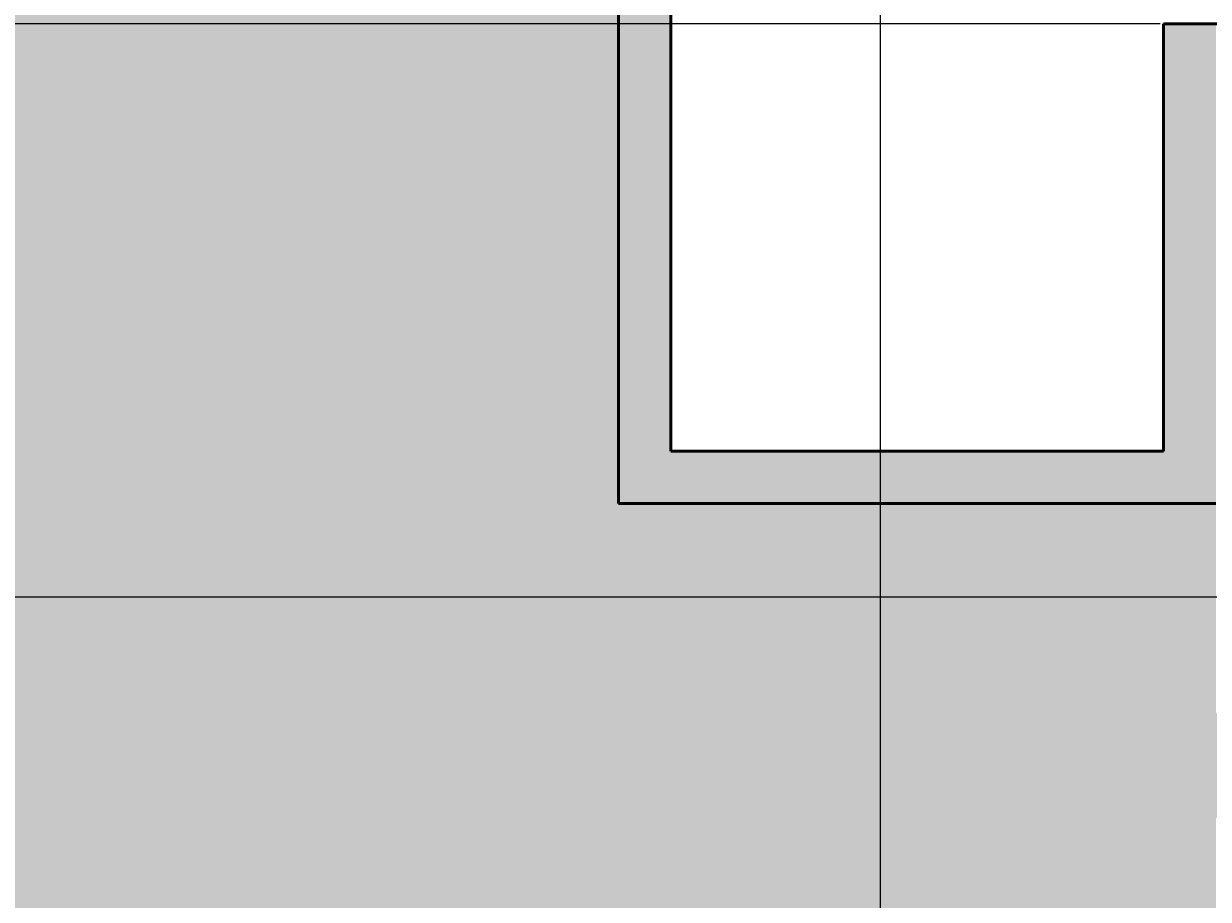
# Model space of a CAD drawing. Units: inches. Extents: x -12 to 334, y -10 to 186.
# Tile 16 of 77: x 42 to 64, y 92 to 109. Entities that reach past the tile are written whole.
import ezdxf

# ---------------------------------------------------------------- set-up
doc = ezdxf.new("R2010")
doc.units = ezdxf.units.IN
doc.header["$MEASUREMENT"] = 0
for name, color, linetype, lineweight in [('M-DIMS', 2, 'Continuous', 18), ('M-EQPM', 7, 'Continuous', 50), ('M-EQPM-PATT', 8, 'Continuous', 18)]:
    doc.layers.add(name, color=color, linetype=linetype, lineweight=lineweight)
doc.styles.get("Standard").update_dxf_attribs({"font": 'arial.ttf'})
doc.dimstyles.get("Standard").update_dxf_attribs({"dimtxt": 0.18, "dimasz": 0.18, "dimexe": 0.18, "dimexo": 0.0625, "dimgap": 0.09, "dimtad": 0, "dimtih": 1, "dimtoh": 1, "dimdec": 4, "dimzin": 0, "dimdsep": 46, "dimtxsty": 'Standard', "dimcen": 0.09, "dimadec": 0, "dimazin": 0, "dimtfac": 1, "dimtdec": 4, "dimtofl": 0, "dimtmove": 0, "dimatfit": 3, "dimfxl": 1, "dimtolj": 1, "dimtzin": 0, "dimarcsym": 0})

# ---------------------------------------------------------------- blocks, each defined once
blk = doc.blocks.new('*D14')
at = {"layer": 'Defpoints', "color": 0, "transparency": 16777216}
for p in [(63.5, 109.058), (-11.174, 49.45), (64.207, 49.45)]:
    blk.add_point(p, dxfattribs=at)
at = {"layer": 'M-DIMS', "color": 0, "lineweight": -2, "transparency": 16777216}
for p, q in [((63.438, 109.058), (-11.354, 109.058)), ((-11.174, 108.878), (-11.174, 79.436)), ((-11.174, 49.63), (-11.174, 79.072)), ((64.144, 49.45), (-11.354, 49.45))]:
    blk.add_line(p, q, dxfattribs=at)
at = {"layer": 'M-DIMS', "color": 0, "transparency": 16777216}
for points in [[(-11.204, 108.878), (-11.144, 108.878), (-11.174, 109.058)], [(-11.204, 49.63), (-11.144, 49.63), (-11.174, 49.45)]]:
    blk.add_solid(points, dxfattribs=at)
at = {"layer": 'M-DIMS', "color": 0, "transparency": 16777216, "insert": (-11.174, 79.254), "char_height": 0.18, "attachment_point": 5}
blk.add_mtext('\\A1;59.61', dxfattribs=at)
blk = doc.blocks.new('*D26')
at = {"layer": 'Defpoints', "color": 0, "transparency": 16777216}
for p in [(87.888, 169.385), (87.888, 56.321), (58.1, 33.675)]:
    blk.add_point(p, dxfattribs=at)
at = {"layer": 'M-DIMS', "color": 0, "lineweight": -2, "transparency": 16777216}
for p, q in [((58.1, 33.738), (58.1, 169.565)), ((87.888, 56.383), (87.888, 169.565)), ((58.28, 169.385), (72.599, 169.385)), ((87.708, 169.385), (73.389, 169.385))]:
    blk.add_line(p, q, dxfattribs=at)
at = {"layer": 'M-DIMS', "color": 0, "transparency": 16777216}
for points in [[(58.28, 169.415), (58.28, 169.355), (58.1, 169.385)], [(87.708, 169.415), (87.708, 169.355), (87.888, 169.385)]]:
    blk.add_solid(points, dxfattribs=at)
at = {"layer": 'M-DIMS', "color": 0, "transparency": 16777216, "insert": (72.994, 169.385), "char_height": 0.18, "attachment_point": 5}
blk.add_mtext('\\A1;29.79', dxfattribs=at)
blk = doc.blocks.new('*D35')
at = {"layer": 'Defpoints', "color": 0, "transparency": 16777216}
for p in [(216.428, 98.108), (-11.174, 61.105), (216.428, 61.105)]:
    blk.add_point(p, dxfattribs=at)
at = {"layer": 'M-DIMS', "color": 0, "lineweight": -2, "transparency": 16777216}
for p, q in [((216.365, 98.108), (-11.354, 98.108)), ((-11.174, 97.928), (-11.174, 79.788)), ((-11.174, 61.285), (-11.174, 79.424)), ((216.365, 61.105), (-11.354, 61.105))]:
    blk.add_line(p, q, dxfattribs=at)
at = {"layer": 'M-DIMS', "color": 0, "transparency": 16777216}
for points in [[(-11.204, 97.928), (-11.144, 97.928), (-11.174, 98.108)], [(-11.204, 61.285), (-11.144, 61.285), (-11.174, 61.105)]]:
    blk.add_solid(points, dxfattribs=at)
at = {"layer": 'M-DIMS', "color": 0, "transparency": 16777216, "insert": (-11.174, 79.606), "char_height": 0.18, "attachment_point": 5}
blk.add_mtext('\\A1;37', dxfattribs=at)

msp = doc.modelspace()

# ---------------------------------------------------------------- hatches: boundary and pattern name
at = {"layer": 'M-EQPM-PATT'}
h = msp.add_hatch(color=256, dxfattribs=at)
h.set_gradient(color1=(99, 100, 102), color2=(99, 100, 102), tint=1)
h.paths.add_polyline_path([(4.3766, 80.754, -0.4132606), (23.5807, 99.8958), (37.1002, 99.8958), (37.1002, 127.7078), (32.1002, 127.7078), (32.1002, 125.2078), (36.1002, 125.2078), (36.1002, 100.8958), (23.5807, 100.8958, 1), (23.5807, 60.4872), (36.1002, 60.4872), (36.1002, 36.1752), (32.1002, 36.1752), (32.1002, 33.6752), (37.1002, 33.6752), (37.1002, 61.4872), (23.5807, 61.4872, -0.384914), (4.4744, 78.754), (72.9244, 78.754), (72.9244, 69.6117), (75.9244, 69.6117), (75.9244, 89.8963), (72.9244, 89.8963), (72.9244, 80.754)])
h.paths.add_polyline_path([(54.1002, 125.2078), (58.1002, 125.2078), (58.1002, 127.7078), (53.1002, 127.7078), (53.1002, 99.8958), (64.5, 99.8958), (64.5, 109.0583), (63.5, 109.0583), (63.5, 100.8958), (54.1002, 100.8958)], flags=17)
h.paths.add_polyline_path([(53.1002, 33.6752), (58.1002, 33.6752), (58.1002, 36.1752), (54.1002, 36.1752), (54.1002, 60.4872), (64.2068, 60.4872), (64.2068, 49.4497), (87.8879, 49.4497), (87.8879, 55.3205), (104.8919, 55.3205), (104.8919, 30.8541), (99.8919, 30.8541), (99.8919, 28.8541), (105.8919, 28.8541), (105.8919, 56.3205), (87.8879, 56.3205), (87.8879, 63.6117), (86.8879, 63.6117), (86.8879, 50.4497), (65.0061, 50.4497), (65.0061, 63.6117), (64.5, 63.6117), (64.5, 61.4872), (53.1002, 61.4872)])
h.paths.add_polyline_path([(121.8919, 28.8541), (121.8919, 30.8541), (116.8919, 30.8541), (116.8919, 45.8541), (209.6965, 45.8541), (209.9204, 46.8541), (115.8919, 46.8541), (115.8919, 28.8541)])
h.paths.add_polyline_path([(221.5761, 32.8541), (216.5761, 32.8541), (216.5761, 30.8541), (222.5761, 30.8541), (222.5761, 46.8541), (209.9204, 46.8541), (209.6965, 45.8541), (221.5761, 45.8541)])
h.paths.add_polyline_path([(233.5761, 45.8541), (249.8485, 45.8541), (249.3759, 46.8541), (232.5761, 46.8541), (232.5761, 30.8541), (238.5761, 30.8541), (238.5761, 32.8541), (233.5761, 32.8541)])
h = msp.add_hatch(color=256, dxfattribs=at)
h.set_gradient(color1=(205, 32, 39), color2=(205, 32, 39), tint=1)
h.paths.add_polyline_path([(64.5, 80.754), (64.5, 89.8963), (226.6083, 89.8963, -1), (226.6083, 69.6117), (64.5, 69.6117), (64.5, 78.754), (4.4744, 78.754, 0.384914), (23.5807, 61.4872), (37.1002, 61.4872), (37.1002, 33.6752), (53.1002, 33.6752), (53.1002, 61.4872), (64.5, 61.4872), (64.5, 63.6117), (226.6083, 63.6117, 1), (226.6083, 95.8963), (64.5, 95.8963), (64.5, 99.8958), (53.1002, 99.8958), (53.1002, 127.7078), (37.1002, 127.7078), (37.1002, 99.8958), (23.5807, 99.8958, 0.4132606), (4.3766, 80.754)])
h.paths.add_polyline_path([(64.5, 91.8963), (64.5, 93.8963), (226.6083, 93.8963, -1), (226.6083, 65.6117), (64.5, 65.6117), (64.5, 67.6117), (226.6083, 67.6117, 1), (226.6083, 91.8963)], flags=16)

# ---------------------------------------------------------------- linework, layer by layer
at = {"layer": 'M-EQPM'}
for p, q in [((53.1002, 99.8958), (53.1002, 127.7078)), ((54.1002, 100.8958), (54.1002, 125.2078)), ((63.5, 109.0583), (86.8879, 109.0583)), ((63.5, 100.8958), (63.5, 109.0583))]:
    msp.add_line(p, q, dxfattribs=at)
for points in [[(54.1002, 100.8958), (63.5, 100.8958)], [(53.1002, 99.8958), (64.5, 99.8958)]]:
    msp.add_lwpolyline(points, dxfattribs=at)

# ---------------------------------------------------------------- dimensions: what is measured, and where the dimension line sits
at = {"layer": 'M-DIMS'}
dim = msp.add_linear_dim(base=(87.8879, 169.3845), p1=(58.1002, 33.6752), p2=(87.8879, 56.3205), dimstyle='Standard', override={"dimdec": 2, "dimlfac": 1, "dimrnd": 0, "dimzin": 0, "dimdsep": 46, "dimlunit": 2}, dxfattribs=at)
dim.commit()
dim.dimension.update_dxf_attribs({"geometry": '*D26', "text_midpoint": (72.9941, 169.3845)})
for base, p1, p2, override, picture, middle in [((-11.1736, 49.4497), (63.5, 109.0583), (64.2068, 49.4497), {"dimdec": 2, "dimlfac": 1, "dimrnd": 0, "dimzin": 0, "dimdsep": 46, "dimlunit": 2}, '*D14', (-11.1735, 79.254)), ((-11.1736, 61.1045), (216.4278, 98.1081), (216.4278, 61.1045), {"dimdec": 0, "dimlfac": 1, "dimrnd": 0, "dimzin": 0, "dimdsep": 46, "dimlunit": 2}, '*D35', (-11.1735, 79.6063))]:
    dim = msp.add_linear_dim(base=base, p1=p1, p2=p2, angle=90, dimstyle='Standard', override=override, dxfattribs=at)
    dim.commit()
    dim.dimension.update_dxf_attribs({"geometry": picture, "text_midpoint": middle})

doc.saveas('drawing.dxf')
